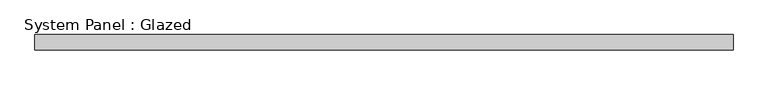
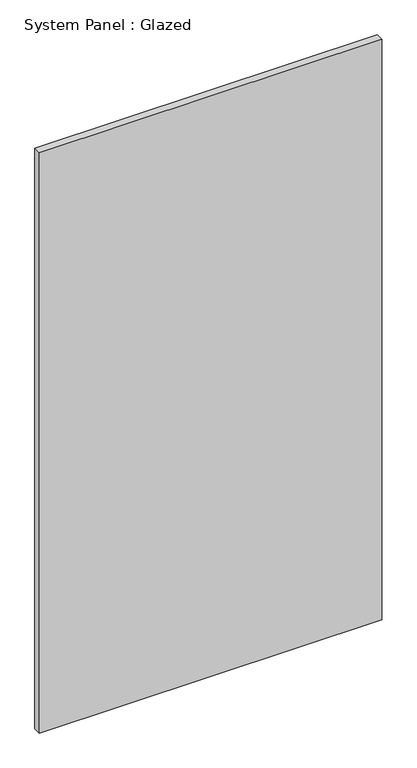
"""IFC4 building model written with IfcOpenShell, lengths in millimetres: plate geometry, System Panel : Glazed."""

from ifc_helpers import new_model, si_unit, origin, origin_with_axes, place, context, project, spatial, polyline, outline, extrude, source, transform, mapped, element, save


def system_panel_glazed_76d7ee11(model_context):
    return source(origin(), model_context, "Body", "SweptSolid", [
        extrude(outline(polyline([(577.85, 19.05), (-577.85, 19.05), (-577.85, 44.45), (577.85, 44.45), (577.85, 19.05)])), origin_with_axes(), (0.0, 0.0, 1.0), 2070.1),
    ])


if __name__ == "__main__":
    model = new_model("IFC4")
    model_context = context("Model", 3, world=origin())
    ifc_project = project(units=[si_unit("LENGTHUNIT", "METRE", prefix="MILLI")], contexts=[model_context])
    site = spatial("IfcSite", under=ifc_project)
    building = spatial("IfcBuilding", under=site)
    placement = place(None, origin())
    system_panel_glazed_shape = system_panel_glazed_76d7ee11(model_context)
    element("IfcPlate", 1, ObjectType="System Panel : Glazed", at=placement, inside=building, context=model_context, shape_type="MappedRepresentation", body=[
        mapped(system_panel_glazed_shape, transform((0.0, 0.0, 0.0), x_axis=(1.0, 0.0, 0.0), y_axis=(0.0, 1.0, 0.0), z_axis=(0.0, 0.0, 1.0))),
    ])
    save(model, "model.ifc")

# Revit data of these elements
# Type "System Panel : Glazed"
#   Construction Type Id = "GSP4R"
#   Analytic Construction = "1/8 in Pilkington single glazing"
#   Visual Light Transmittance = 0.9
#   Solar Heat Gain Coefficient = 0.86
#   Heat Transfer Coefficient (U) = 1.18115 BTU/(h·ft²·°F)
#   Define Thermal Properties by = 1
# Element 1 (IfcPlate, "System Panel : Glazed")
#   Materials on its faces: "Glass"
# Materials
#   "Glass": class "Glass", colour RGB 0 128 192, transparency 0.75, Description = "Soda Lime Glass", Cost = 0
